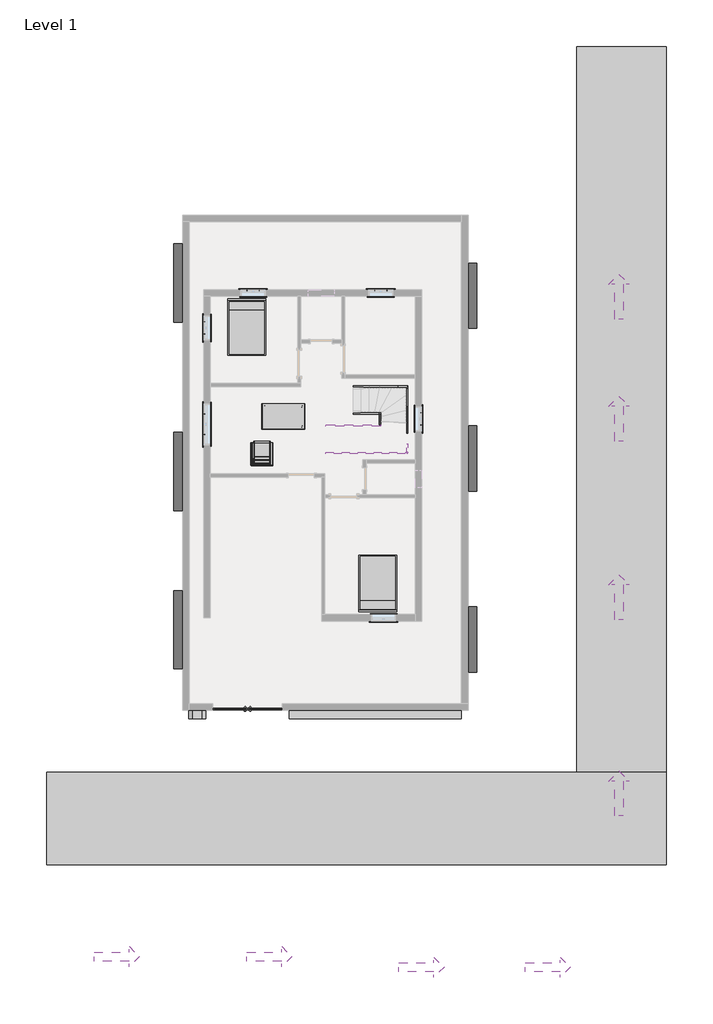
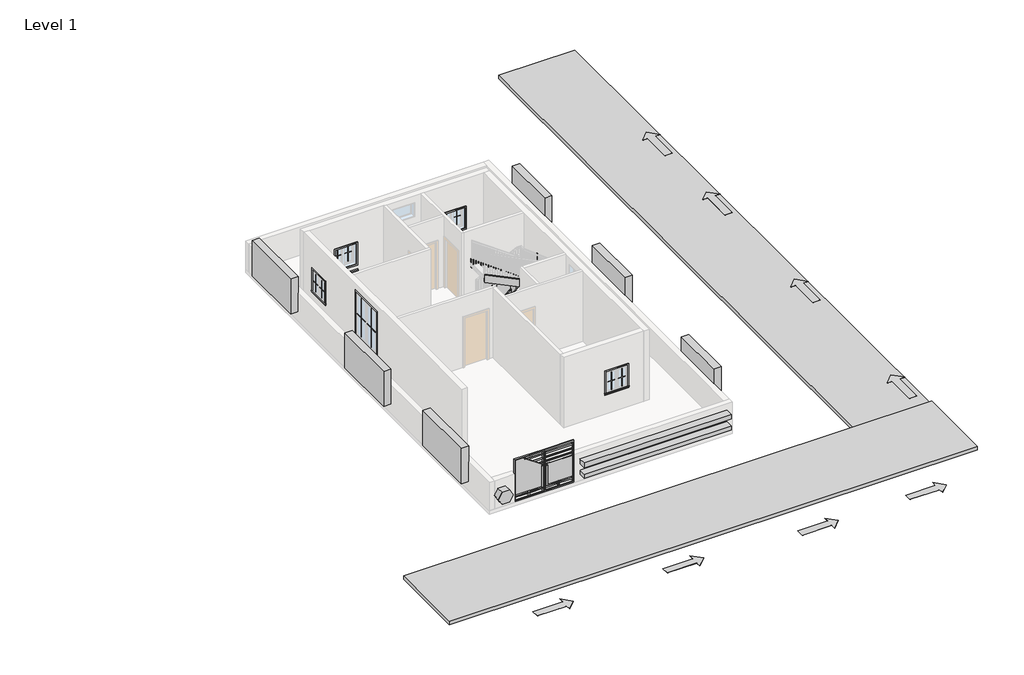
# One storey, part 3 of 3: 30 proxies, 9 members, 8 geographic elements, 4 furniture elements.
"""IFC4 building model written with IfcOpenShell, lengths in millimetres."""

from ifc_helpers import new_model, si_unit, frame, origin, place, context, project, spatial, polyline, outline, extrude, transform, mapped, element, save
from components import generic_models_113f6068, generic_models_1_generic_models_1_a47648ae, generic_models_2_generic_models_2_4eaefd90, generic_models_3_generic_models_3_d2748d51, generic_models_4_generic_models_4_994ceaf2, generic_models_5_generic_models_5_1652e53f, muntin_pattern_2x2_muntin_pattern_2x2_b3fe6957, muntin_pattern_2x2_muntin_pattern_2x2_3e0ecaf2, muntin_pattern_2x2_muntin_pattern_2x2_bff912c5, muntin_pattern_2x2_muntin_pattern_2x2_c2194282, trim_window_exterior_flat_with_sill_41619996, trim_window_exterior_flat_with_sill_e04b3088, trim_window_interior_flat_picture_frame_51c85655, trim_window_interior_flat_picture_frame_2a7685fe, furniture_f28dd14e, furniture_402a1f5e, bed_17739_bed_17739_15c61121, dining_table_14755_dining_table_14755_d89cb775, direction_arrows_straight_direction_arrow_straight_a0d3235c

model = new_model("IFC4")

# Units and contexts
model_context = context("Model", 3, world=origin())
ifc_project = project(units=[si_unit("LENGTHUNIT", "METRE", prefix="MILLI")], contexts=[model_context])

# Site, building, storey
site = spatial("IfcSite", under=ifc_project)
building = spatial("IfcBuilding", under=site)
storey = spatial("IfcBuildingStorey", under=building, Name="Level 1", Elevation=0.0)

# Proxies
placement = place(None, origin())
generic_models_shape = generic_models_113f6068(model_context)
element("IfcBuildingElementProxy", 1, Name="Generic Models", at=placement, inside=storey, context=model_context, shape_type="MappedRepresentation", body=[
    mapped(generic_models_shape, transform((-3534.8915084, -8307.1830082, 0.0), x_axis=(1.0, 0.0, 0.0), y_axis=(0.0, 1.0, 0.0), z_axis=(0.0, 0.0, 1.0))),
])
generic_models_1_generic_models_1_shape = generic_models_1_generic_models_1_a47648ae(model_context)
element("IfcBuildingElementProxy", 2, Name="Generic Models 1 : Generic Models 1", ObjectType="Generic Models 1 : Generic Models 1", at=placement, inside=storey, context=model_context, shape_type="MappedRepresentation", body=[
    mapped(generic_models_1_generic_models_1_shape, transform((0.0, 0.0, 0.0), x_axis=(1.0, 0.0, 0.0), y_axis=(0.0, 1.0, 0.0), z_axis=(0.0, 0.0, 1.0))),
])
generic_models_2_generic_models_2_shape = generic_models_2_generic_models_2_4eaefd90(model_context)
element("IfcBuildingElementProxy", 3, Name="Generic Models 2 : Generic Models 2", ObjectType="Generic Models 2 : Generic Models 2", at=placement, inside=storey, context=model_context, shape_type="MappedRepresentation", body=[
    mapped(generic_models_2_generic_models_2_shape, transform((0.0, 0.0, 0.0), x_axis=(1.0, 0.0, 0.0), y_axis=(0.0, 1.0, 0.0), z_axis=(0.0, 0.0, 1.0))),
])
generic_models_3_generic_models_3_shape = generic_models_3_generic_models_3_d2748d51(model_context)
element("IfcBuildingElementProxy", 4, Name="Generic Models 3 : Generic Models 3", ObjectType="Generic Models 3 : Generic Models 3", at=placement, inside=storey, context=model_context, shape_type="MappedRepresentation", body=[
    mapped(generic_models_3_generic_models_3_shape, transform((0.0, 0.0, 0.0), x_axis=(1.0, 0.0, 0.0), y_axis=(0.0, 1.0, 0.0), z_axis=(0.0, 0.0, 1.0))),
])
generic_models_4_generic_models_4_shape = generic_models_4_generic_models_4_994ceaf2(model_context)
element("IfcBuildingElementProxy", 5, Name="Generic Models 4 : Generic Models 4", ObjectType="Generic Models 4 : Generic Models 4", at=placement, inside=storey, context=model_context, shape_type="MappedRepresentation", body=[
    mapped(generic_models_4_generic_models_4_shape, transform((0.0, 0.0, 0.0), x_axis=(1.0, 0.0, 0.0), y_axis=(0.0, 1.0, 0.0), z_axis=(0.0, 0.0, 1.0))),
])
generic_models_5_generic_models_5_shape = generic_models_5_generic_models_5_1652e53f(model_context)
element("IfcBuildingElementProxy", 6, Name="Generic Models 5 : Generic Models 5", ObjectType="Generic Models 5 : Generic Models 5", at=placement, inside=storey, context=model_context, shape_type="MappedRepresentation", body=[
    mapped(generic_models_5_generic_models_5_shape, transform((0.0, 0.0, 0.0), x_axis=(1.0, 0.0, 0.0), y_axis=(0.0, 1.0, 0.0), z_axis=(0.0, 0.0, 1.0))),
])
muntin_pattern_2x2_muntin_pattern_2x2_shape = muntin_pattern_2x2_muntin_pattern_2x2_b3fe6957(model_context)
element("IfcBuildingElementProxy", 7, Name="Muntin Pattern_2x2 : Muntin Pattern_2x2", ObjectType="Muntin Pattern_2x2 : Muntin Pattern_2x2", at=placement, inside=storey, context=model_context, shape_type="MappedRepresentation", body=[
    mapped(muntin_pattern_2x2_muntin_pattern_2x2_shape, transform((-3555.5290084, 6319.8685985, 984.25), x_axis=(1.0, 0.0, 0.0), y_axis=(0.0, 1.0, 0.0), z_axis=(0.0, 0.0, 1.0))),
])
element("IfcBuildingElementProxy", 8, Name="Muntin Pattern_2x2 : Muntin Pattern_2x2", ObjectType="Muntin Pattern_2x2 : Muntin Pattern_2x2", at=placement, inside=storey, context=model_context, shape_type="MappedRepresentation", body=[
    mapped(muntin_pattern_2x2_muntin_pattern_2x2_shape, transform((1435.5709916, -5243.4814015, 984.25), x_axis=(-1.0, 0.0, 0.0), y_axis=(0.0, -1.0, 0.0), z_axis=(0.0, 0.0, 1.0))),
])
element("IfcBuildingElementProxy", 9, Name="Muntin Pattern_2x2 : Muntin Pattern_2x2", ObjectType="Muntin Pattern_2x2 : Muntin Pattern_2x2", at=placement, inside=storey, context=model_context, shape_type="MappedRepresentation", body=[
    mapped(muntin_pattern_2x2_muntin_pattern_2x2_shape, transform((2545.2334916, 2028.8560985, 984.25), x_axis=(0.0, -1.0, 0.0), y_axis=(1.0, 0.0, 0.0), z_axis=(0.0, 0.0, 1.0))),
])
element("IfcBuildingElementProxy", 10, Name="Muntin Pattern_2x2 : Muntin Pattern_2x2", ObjectType="Muntin Pattern_2x2 : Muntin Pattern_2x2", at=placement, inside=storey, context=model_context, shape_type="MappedRepresentation", body=[
    mapped(muntin_pattern_2x2_muntin_pattern_2x2_shape, transform((908.5209916, 6319.8685985, 984.25), x_axis=(1.0, 0.0, 0.0), y_axis=(0.0, 1.0, 0.0), z_axis=(0.0, 0.0, 1.0))),
])
element("IfcBuildingElementProxy", 11, Name="Muntin Pattern_2x2 : Muntin Pattern_2x2", ObjectType="Muntin Pattern_2x2 : Muntin Pattern_2x2", at=placement, inside=storey, context=model_context, shape_type="MappedRepresentation", body=[
    mapped(muntin_pattern_2x2_muntin_pattern_2x2_shape, transform((-5055.7165084, 4781.5810985, 984.25), x_axis=(0.0, 1.0, 0.0), y_axis=(-1.0, 0.0, 0.0), z_axis=(0.0, 0.0, 1.0))),
])
muntin_pattern_2x2_muntin_pattern_2x2_2_shape = muntin_pattern_2x2_muntin_pattern_2x2_3e0ecaf2(model_context)
element("IfcBuildingElementProxy", 12, Name="Muntin Pattern_2x2 : Muntin Pattern_2x2", ObjectType="Muntin Pattern_2x2 : Muntin Pattern_2x2", at=placement, inside=storey, context=model_context, shape_type="MappedRepresentation", body=[
    mapped(muntin_pattern_2x2_muntin_pattern_2x2_2_shape, transform((-3126.9040084, 6319.8685985, 984.25), x_axis=(-1.0, 0.0, 0.0), y_axis=(0.0, -1.0, 0.0), z_axis=(0.0, 0.0, 1.0))),
])
element("IfcBuildingElementProxy", 13, Name="Muntin Pattern_2x2 : Muntin Pattern_2x2", ObjectType="Muntin Pattern_2x2 : Muntin Pattern_2x2", at=placement, inside=storey, context=model_context, shape_type="MappedRepresentation", body=[
    mapped(muntin_pattern_2x2_muntin_pattern_2x2_2_shape, transform((1006.9459916, -5243.4814015, 984.25), x_axis=(1.0, 0.0, 0.0), y_axis=(0.0, 1.0, 0.0), z_axis=(0.0, 0.0, 1.0))),
])
element("IfcBuildingElementProxy", 14, Name="Muntin Pattern_2x2 : Muntin Pattern_2x2", ObjectType="Muntin Pattern_2x2 : Muntin Pattern_2x2", at=placement, inside=storey, context=model_context, shape_type="MappedRepresentation", body=[
    mapped(muntin_pattern_2x2_muntin_pattern_2x2_2_shape, transform((2545.2334916, 1600.2310985, 984.25), x_axis=(0.0, 1.0, 0.0), y_axis=(-1.0, 0.0, 0.0), z_axis=(0.0, 0.0, 1.0))),
])
element("IfcBuildingElementProxy", 15, Name="Muntin Pattern_2x2 : Muntin Pattern_2x2", ObjectType="Muntin Pattern_2x2 : Muntin Pattern_2x2", at=placement, inside=storey, context=model_context, shape_type="MappedRepresentation", body=[
    mapped(muntin_pattern_2x2_muntin_pattern_2x2_2_shape, transform((1337.1459916, 6319.8685985, 984.25), x_axis=(-1.0, 0.0, 0.0), y_axis=(0.0, -1.0, 0.0), z_axis=(0.0, 0.0, 1.0))),
])
element("IfcBuildingElementProxy", 16, Name="Muntin Pattern_2x2 : Muntin Pattern_2x2", ObjectType="Muntin Pattern_2x2 : Muntin Pattern_2x2", at=placement, inside=storey, context=model_context, shape_type="MappedRepresentation", body=[
    mapped(muntin_pattern_2x2_muntin_pattern_2x2_2_shape, transform((-5055.7165084, 5210.2060985, 984.25), x_axis=(0.0, -1.0, 0.0), y_axis=(1.0, 0.0, 0.0), z_axis=(0.0, 0.0, 1.0))),
])
muntin_pattern_2x2_muntin_pattern_2x2_3_shape = muntin_pattern_2x2_muntin_pattern_2x2_bff912c5(model_context)
element("IfcBuildingElementProxy", 17, Name="Muntin Pattern_2x2 : Muntin Pattern_2x2", ObjectType="Muntin Pattern_2x2 : Muntin Pattern_2x2", at=placement, inside=storey, context=model_context, shape_type="MappedRepresentation", body=[
    mapped(muntin_pattern_2x2_muntin_pattern_2x2_3_shape, transform((-5055.7165084, 1263.6810985, 984.25), x_axis=(0.0, 1.0, 0.0), y_axis=(-1.0, 0.0, 0.0), z_axis=(0.0, 0.0, 1.0))),
])
muntin_pattern_2x2_muntin_pattern_2x2_4_shape = muntin_pattern_2x2_muntin_pattern_2x2_c2194282(model_context)
element("IfcBuildingElementProxy", 18, Name="Muntin Pattern_2x2 : Muntin Pattern_2x2", ObjectType="Muntin Pattern_2x2 : Muntin Pattern_2x2", at=placement, inside=storey, context=model_context, shape_type="MappedRepresentation", body=[
    mapped(muntin_pattern_2x2_muntin_pattern_2x2_4_shape, transform((-5055.7165084, 1984.4060985, 984.25), x_axis=(0.0, -1.0, 0.0), y_axis=(1.0, 0.0, 0.0), z_axis=(0.0, 0.0, 1.0))),
])
trim_window_exterior_flat_with_sill_shape = trim_window_exterior_flat_with_sill_41619996(model_context)
element("IfcBuildingElementProxy", 19, Name="Trim-Window-Exterior-Flat : with Sill", ObjectType="Trim-Window-Exterior-Flat : with Sill", at=placement, inside=storey, context=model_context, shape_type="MappedRepresentation", body=[
    mapped(trim_window_exterior_flat_with_sill_shape, transform((-3341.2165084, 6329.3935985, 1828.8), x_axis=(-1.0, 0.0, 0.0), y_axis=(0.0, 0.0, 1.0), z_axis=(0.0, 1.0, 0.0))),
])
element("IfcBuildingElementProxy", 20, Name="Trim-Window-Exterior-Flat : with Sill", ObjectType="Trim-Window-Exterior-Flat : with Sill", at=placement, inside=storey, context=model_context, shape_type="MappedRepresentation", body=[
    mapped(trim_window_exterior_flat_with_sill_shape, transform((1221.2584916, -5253.0064015, 1828.8), x_axis=(1.0, 0.0, 0.0), y_axis=(0.0, 0.0, 1.0), z_axis=(0.0, -1.0, 0.0))),
])
element("IfcBuildingElementProxy", 21, Name="Trim-Window-Exterior-Flat : with Sill", ObjectType="Trim-Window-Exterior-Flat : with Sill", at=placement, inside=storey, context=model_context, shape_type="MappedRepresentation", body=[
    mapped(trim_window_exterior_flat_with_sill_shape, transform((2554.7584916, 1814.5435985, 1828.8), x_axis=(0.0, 1.0, 0.0), y_axis=(0.0, 0.0, 1.0), z_axis=(1.0, 0.0, 0.0))),
])
element("IfcBuildingElementProxy", 22, Name="Trim-Window-Exterior-Flat : with Sill", ObjectType="Trim-Window-Exterior-Flat : with Sill", at=placement, inside=storey, context=model_context, shape_type="MappedRepresentation", body=[
    mapped(trim_window_exterior_flat_with_sill_shape, transform((1122.8334916, 6329.3935985, 1828.8), x_axis=(-1.0, 0.0, 0.0), y_axis=(0.0, 0.0, 1.0), z_axis=(0.0, 1.0, 0.0))),
])
element("IfcBuildingElementProxy", 23, Name="Trim-Window-Exterior-Flat : with Sill", ObjectType="Trim-Window-Exterior-Flat : with Sill", at=placement, inside=storey, context=model_context, shape_type="MappedRepresentation", body=[
    mapped(trim_window_exterior_flat_with_sill_shape, transform((-5065.2415084, 4995.8935985, 1828.8), x_axis=(0.0, -1.0, 0.0), y_axis=(0.0, 0.0, 1.0), z_axis=(-1.0, 0.0, 0.0))),
])
trim_window_exterior_flat_with_sill_2_shape = trim_window_exterior_flat_with_sill_e04b3088(model_context)
element("IfcBuildingElementProxy", 24, Name="Trim-Window-Exterior-Flat : with Sill", ObjectType="Trim-Window-Exterior-Flat : with Sill", at=placement, inside=storey, context=model_context, shape_type="MappedRepresentation", body=[
    mapped(trim_window_exterior_flat_with_sill_2_shape, transform((-5065.2415084, 1624.0435985, 2743.2), x_axis=(0.0, -1.0, 0.0), y_axis=(0.0, 0.0, 1.0), z_axis=(-1.0, 0.0, 0.0))),
])
trim_window_interior_flat_picture_frame_shape = trim_window_interior_flat_picture_frame_51c85655(model_context)
element("IfcBuildingElementProxy", 25, Name="Trim-Window-Interior-Flat : Picture Frame", ObjectType="Trim-Window-Interior-Flat : Picture Frame", at=placement, inside=storey, context=model_context, shape_type="MappedRepresentation", body=[
    mapped(trim_window_interior_flat_picture_frame_shape, transform((-3341.2165084, 6100.7935985, 1828.8), x_axis=(1.0, 0.0, 0.0), y_axis=(0.0, 0.0, 1.0), z_axis=(0.0, -1.0, 0.0))),
])
element("IfcBuildingElementProxy", 26, Name="Trim-Window-Interior-Flat : Picture Frame", ObjectType="Trim-Window-Interior-Flat : Picture Frame", at=placement, inside=storey, context=model_context, shape_type="MappedRepresentation", body=[
    mapped(trim_window_interior_flat_picture_frame_shape, transform((1221.2584916, -5024.4064015, 1828.8), x_axis=(-1.0, 0.0, 0.0), y_axis=(0.0, 0.0, 1.0), z_axis=(0.0, 1.0, 0.0))),
])
element("IfcBuildingElementProxy", 27, Name="Trim-Window-Interior-Flat : Picture Frame", ObjectType="Trim-Window-Interior-Flat : Picture Frame", at=placement, inside=storey, context=model_context, shape_type="MappedRepresentation", body=[
    mapped(trim_window_interior_flat_picture_frame_shape, transform((2326.1584916, 1814.5435985, 1828.8), x_axis=(0.0, -1.0, 0.0), y_axis=(0.0, 0.0, 1.0), z_axis=(-1.0, 0.0, 0.0))),
])
element("IfcBuildingElementProxy", 28, Name="Trim-Window-Interior-Flat : Picture Frame", ObjectType="Trim-Window-Interior-Flat : Picture Frame", at=placement, inside=storey, context=model_context, shape_type="MappedRepresentation", body=[
    mapped(trim_window_interior_flat_picture_frame_shape, transform((1122.8334916, 6100.7935985, 1828.8), x_axis=(1.0, 0.0, 0.0), y_axis=(0.0, 0.0, 1.0), z_axis=(0.0, -1.0, 0.0))),
])
element("IfcBuildingElementProxy", 29, Name="Trim-Window-Interior-Flat : Picture Frame", ObjectType="Trim-Window-Interior-Flat : Picture Frame", at=placement, inside=storey, context=model_context, shape_type="MappedRepresentation", body=[
    mapped(trim_window_interior_flat_picture_frame_shape, transform((-4836.6415084, 4995.8935985, 1828.8), x_axis=(0.0, 1.0, 0.0), y_axis=(0.0, 0.0, 1.0), z_axis=(1.0, 0.0, 0.0))),
])
trim_window_interior_flat_picture_frame_2_shape = trim_window_interior_flat_picture_frame_2a7685fe(model_context)
element("IfcBuildingElementProxy", 30, Name="Trim-Window-Interior-Flat : Picture Frame", ObjectType="Trim-Window-Interior-Flat : Picture Frame", at=placement, inside=storey, context=model_context, shape_type="MappedRepresentation", body=[
    mapped(trim_window_interior_flat_picture_frame_2_shape, transform((-4836.6415084, 1624.0435985, 2743.2), x_axis=(0.0, 1.0, 0.0), y_axis=(0.0, 0.0, 1.0), z_axis=(1.0, 0.0, 0.0))),
])

# Furniture
furniture_shape = furniture_f28dd14e(model_context)
furniture_2_shape = furniture_402a1f5e(model_context)
element("IfcFurniture", 31, at=placement, inside=storey, context=model_context, shape_type="MappedRepresentation", body=[
    mapped(furniture_shape, transform((-3032.3877006, 981.9349825, 0.0), x_axis=(-1.0, 0.0, 0.0), y_axis=(0.0, -1.0, 0.0), z_axis=(0.0, 0.0, 1.0))),
    mapped(furniture_2_shape, transform((-3032.3877006, 981.9349825, 0.0), x_axis=(-1.0, 0.0, 0.0), y_axis=(0.0, -1.0, 0.0), z_axis=(0.0, 0.0, 1.0))),
])
bed_17739_bed_17739_shape = bed_17739_bed_17739_15c61121(model_context)
element("IfcFurniture", 32, ObjectType="Bed_17739 : Bed_17739", at=placement, inside=storey, context=model_context, shape_type="MappedRepresentation", body=[
    mapped(bed_17739_bed_17739_shape, transform((-3560.2915084, 4995.8935985, 0.0), x_axis=(1.0, 0.0, 0.0), y_axis=(0.0, 1.0, 0.0), z_axis=(0.0, 0.0, 1.0))),
])
element("IfcFurniture", 33, ObjectType="Bed_17739 : Bed_17739", at=placement, inside=storey, context=model_context, shape_type="MappedRepresentation", body=[
    mapped(bed_17739_bed_17739_shape, transform((1011.7084916, -3919.5064015, 0.0), x_axis=(-1.0, 0.0, 0.0), y_axis=(0.0, -1.0, 0.0), z_axis=(0.0, 0.0, 1.0))),
])
dining_table_14755_dining_table_14755_shape = dining_table_14755_dining_table_14755_d89cb775(model_context)
element("IfcFurniture", 34, ObjectType="Dining_table_14755 : Dining_table_14755", at=placement, inside=storey, context=model_context, shape_type="MappedRepresentation", body=[
    mapped(dining_table_14755_dining_table_14755_shape, transform((-3032.3877006, 1444.8879061, 0.0), x_axis=(1.0, 0.0, 0.0), y_axis=(0.0, 1.0, 0.0), z_axis=(0.0, 0.0, 1.0))),
])

# Geographic elements
direction_arrows_straight_direction_arrow_straight_shape = direction_arrows_straight_direction_arrow_straight_a0d3235c(model_context)
element("IfcGeographicElement", 35, ObjectType="Direction Arrows - Straight : Direction Arrow - Straight", at=placement, inside=storey, context=model_context, shape_type="MappedRepresentation", body=[
    mapped(direction_arrows_straight_direction_arrow_straight_shape, transform((-8896.9922047, -16987.8064015, 1828.8), x_axis=(0.0, -1.0, 0.0), y_axis=(1.0, 0.0, 0.0), z_axis=(0.0, 0.0, 1.0))),
])
element("IfcGeographicElement", 36, ObjectType="Direction Arrows - Straight : Direction Arrow - Straight", at=placement, inside=storey, context=model_context, shape_type="MappedRepresentation", body=[
    mapped(direction_arrows_straight_direction_arrow_straight_shape, transform((-3562.9922047, -16987.8064015, 1828.8), x_axis=(0.0, -1.0, 0.0), y_axis=(1.0, 0.0, 0.0), z_axis=(0.0, 0.0, 1.0))),
])
element("IfcGeographicElement", 37, ObjectType="Direction Arrows - Straight : Direction Arrow - Straight", at=placement, inside=storey, context=model_context, shape_type="MappedRepresentation", body=[
    mapped(direction_arrows_straight_direction_arrow_straight_shape, transform((1758.0144394, -17359.8874325, 1828.8), x_axis=(0.0, -1.0, 0.0), y_axis=(1.0, 0.0, 0.0), z_axis=(0.0, 0.0, 1.0))),
])
element("IfcGeographicElement", 38, ObjectType="Direction Arrows - Straight : Direction Arrow - Straight", at=placement, inside=storey, context=model_context, shape_type="MappedRepresentation", body=[
    mapped(direction_arrows_straight_direction_arrow_straight_shape, transform((6177.6144394, -17359.8874325, 1828.8), x_axis=(0.0, -1.0, 0.0), y_axis=(1.0, 0.0, 0.0), z_axis=(0.0, 0.0, 1.0))),
])
element("IfcGeographicElement", 39, ObjectType="Direction Arrows - Straight : Direction Arrow - Straight", at=placement, inside=storey, context=model_context, shape_type="MappedRepresentation", body=[
    mapped(direction_arrows_straight_direction_arrow_straight_shape, transform((9447.5076868, -12069.3629782, 1828.8), x_axis=(1.0, 0.0, 0.0), y_axis=(0.0, 1.0, 0.0), z_axis=(0.0, 0.0, 1.0))),
])
element("IfcGeographicElement", 40, ObjectType="Direction Arrows - Straight : Direction Arrow - Straight", at=placement, inside=storey, context=model_context, shape_type="MappedRepresentation", body=[
    mapped(direction_arrows_straight_direction_arrow_straight_shape, transform((9447.5076868, -5211.3629782, 1828.8), x_axis=(1.0, 0.0, 0.0), y_axis=(0.0, 1.0, 0.0), z_axis=(0.0, 0.0, 1.0))),
])
element("IfcGeographicElement", 41, ObjectType="Direction Arrows - Straight : Direction Arrow - Straight", at=placement, inside=storey, context=model_context, shape_type="MappedRepresentation", body=[
    mapped(direction_arrows_straight_direction_arrow_straight_shape, transform((9447.5076868, 1037.0370218, 1828.8), x_axis=(1.0, 0.0, 0.0), y_axis=(0.0, 1.0, 0.0), z_axis=(0.0, 0.0, 1.0))),
])
element("IfcGeographicElement", 42, ObjectType="Direction Arrows - Straight : Direction Arrow - Straight", at=placement, inside=storey, context=model_context, shape_type="MappedRepresentation", body=[
    mapped(direction_arrows_straight_direction_arrow_straight_shape, transform((9447.5076868, 5304.2370218, 1828.8), x_axis=(1.0, 0.0, 0.0), y_axis=(0.0, 1.0, 0.0), z_axis=(0.0, 0.0, 1.0))),
])

# Members
element("IfcMember", 43, ObjectType="Stringer - 2\" Width", at=placement, inside=storey, context=model_context, shape_type="SweptSolid", body=[
    extrude(outline(polyline([(239.4504763, 158.6923968), (0.0, 158.6923968), (0.0, 366.2169505), (626.2639814, 1705.9967367), (962.7193197, 1705.9967367), (239.4504763, 158.6923968)])), frame((0.0, 2922.8476133, 0.0), z_axis=(0.0, 1.0, 0.0), x_axis=(0.0, 0.0, 1.0)), (0.0, 0.0, 1.0), 50.8),
])
element("IfcMember", 44, ObjectType="Stringer - 2\" Width", at=placement, inside=storey, context=model_context, shape_type="SweptSolid", body=[
    extrude(outline(polyline([(1705.9967367, 2922.8476133), (1705.9967367, 2973.6476133), (2072.9441983, 2973.6476133), (2022.1441983, 2922.8476133), (1705.9967367, 2922.8476133)])), frame((0.0, 0.0, 626.2639814), z_axis=(0.0, 0.0, 1.0), x_axis=(1.0, 0.0, 0.0)), (0.0, 0.0, 1.0), 336.4553383),
])
element("IfcMember", 45, ObjectType="Stringer - 2\" Width", at=placement, inside=storey, context=model_context, shape_type="SweptSolid", body=[
    extrude(outline(polyline([(2022.1441983, 2922.8476133), (2072.9441983, 2973.6476133), (2072.9441983, 2883.4348143), (2022.1441983, 2883.4348143), (2022.1441983, 2922.8476133)])), frame((0.0, 0.0, 626.2639814), z_axis=(0.0, 0.0, 1.0), x_axis=(1.0, 0.0, 0.0)), (0.0, 0.0, 1.0), 336.4553383),
])
element("IfcMember", 46, ObjectType="Stringer - 2\" Width", at=placement, inside=storey, context=model_context, shape_type="SweptSolid", body=[
    extrude(outline(polyline([(2883.4348143, 962.7193197), (2883.4348143, 626.2639814), (947.0260734, 1335.6990218), (947.0260734, 1672.1543601), (2883.4348143, 962.7193197)])), frame((2022.1441983, 0.0, 0.0), z_axis=(1.0, 0.0, 0.0), x_axis=(0.0, 1.0, 0.0)), (0.0, 0.0, 1.0), 50.8),
])
element("IfcMember", 47, ObjectType="Stringer - 2\" Width", at=placement, inside=storey, context=model_context, shape_type="SweptSolid", body=[
    extrude(outline(polyline([(2022.1441983, 947.0260734), (2072.9441983, 947.0260734), (2072.9441983, 652.4935985), (2022.1441983, 652.4935985), (2022.1441983, 947.0260734)])), frame((0.0, 0.0, 1341.3754285), z_axis=(0.0, 0.0, 1.0), x_axis=(1.0, 0.0, 0.0)), (0.0, 0.0, 1.0), 324.6119022),
])
element("IfcMember", 48, ObjectType="Stringer - 2\" Width", at=placement, inside=storey, context=model_context, shape_type="SweptSolid", body=[
    extrude(outline(polyline([(174.4551137, 158.6923968), (0.0, 158.6923968), (0.0, 426.0767146), (534.1870321, 1072.5901835), (929.5706215, 1072.5901835), (174.4551137, 158.6923968)])), frame((0.0, 1973.2935985, 0.0), z_axis=(0.0, 1.0, 0.0), x_axis=(0.0, 0.0, 1.0)), (0.0, 0.0, 1.0), 50.8),
])
element("IfcMember", 49, ObjectType="Stringer - 2\" Width", at=placement, inside=storey, context=model_context, shape_type="SweptSolid", body=[
    extrude(outline(polyline([(2024.0935985, 1132.896008), (2024.0935985, 630.1724164), (1602.0476133, 1183.7407029), (1602.0476133, 1686.4642945), (2024.0935985, 1132.896008)])), frame((1072.5901835, 0.0, 0.0), z_axis=(1.0, 0.0, 0.0), x_axis=(0.0, 1.0, 0.0)), (0.0, 0.0, 1.0), 50.8),
])
element("IfcMember", 50, ObjectType="Stringer - 2\" Width", at=placement, inside=storey, context=model_context, shape_type="SweptSolid", body=[
    extrude(outline(polyline([(1362.1113348, 1123.3901835), (1739.0379401, 1123.3901835), (3137.1009734, -798.3242294), (2760.1743681, -798.3242294), (1362.1113348, 1123.3901835)])), frame((0.0, 1551.2476133, 0.0), z_axis=(0.0, 1.0, 0.0), x_axis=(0.0, 0.0, 1.0)), (0.0, 0.0, 1.0), 50.8),
])
element("IfcMember", 51, ObjectType="Stringer - 2\" Width", at=placement, inside=storey, context=model_context, shape_type="SweptSolid", body=[
    extrude(outline(polyline([(1361.1873308, 2072.9441983), (1641.2397747, 2072.9441983), (3039.9971818, -798.3242294), (2715.3852796, -798.3242294), (1361.1873308, 1981.4757528), (1361.1873308, 2072.9441983)])), frame((0.0, 601.6935985, 0.0), z_axis=(0.0, 1.0, 0.0), x_axis=(0.0, 0.0, 1.0)), (0.0, 0.0, 1.0), 50.8),
])

save(model, "model.ifc")

# Revit data of these elements
# Type
#   sheet = none
#   pipe = none
#   handal = none
#   faram = none
#   Default Elevation = 0
# Type "Muntin Pattern_2x2 : Muntin Pattern_2x2"
#   Width [instance default] = 4' - 0"
#   Thickness = 0' - 0 1/2"
#   Height [instance default] = 4' - 0"
#   Distance = 0' - 0 3/4"
#   Interior Material [instance default] = none
#   Exterior Material [instance default] = none
#   Default Elevation = 0
# Type "Trim-Window-Exterior-Flat : with Sill"
#   Trim Width = 0' - 2 1/4"
#   Trim Thickness_Picture Frame = 0' - 1 1/4"
#   Trim Thickness_with Sill = 0' - 0 3/4"
#   Sill Thickness = 0' - 1 1/4"
#   Opening Width [instance default] = 2' - 0"
#   Opening Height [instance default] = 3' - 0"
#   Default Elevation = 4' - 0"
#   Sill = yes
#   Picture Frame = no
#   Trim Material [instance default] = none
# Type "Trim-Window-Interior-Flat : Picture Frame"
#   Trim Thickness_Picture Frame = 0' - 1 1/4"
#   Trim Width = 0' - 2 1/4"
#   Trim Thickness_with Sill = 0' - 0 3/4"
#   Sill Thickness = 0' - 1 1/4"
#   Opening Width [instance default] = 2' - 0"
#   Opening Height [instance default] = 3' - 0"
#   Default Elevation = 4' - 0"
#   Sill = no
#   Picture Frame = yes
#   Trim Material [instance default] = none
# Type
#   Width [instance] = 2' - 6.31496"
#   Default Elevation = 0
# Type "Bed_17739 : Bed_17739"
#   Default Elevation = 0
# Type "Dining_table_14755 : Dining_table_14755"
#   Lengte [instance default] = 4' - 11.05512"
#   Breedte [instance default] = 2' - 11.43307"
#   Tafelblad = none
#   Poten = none
#   Default Elevation = 0
# Element 1 (IfcBuildingElementProxy)
#   Phase Created = New Construction
# Element 2 (IfcBuildingElementProxy, "Generic Models 1 : Generic Models 1")
#   Phase Created = New Construction
#   Materials on its faces: "Wood - Stained", "Softwood, Lumber"
# Element 3 (IfcBuildingElementProxy, "Generic Models 2 : Generic Models 2")
#   Phase Created = New Construction
#   Materials on its faces: "Wood - Stained"
# Element 4 (IfcBuildingElementProxy, "Generic Models 3 : Generic Models 3")
#   Phase Created = New Construction
#   Materials on its faces: "Parking Stripe"
# Element 5 (IfcBuildingElementProxy, "Generic Models 4 : Generic Models 4")
#   Phase Created = New Construction
#   Materials on its faces: "Parking Stripe"
# Element 6 (IfcBuildingElementProxy, "Generic Models 5 : Generic Models 5")
#   Phase Created = New Construction
# Elements 7, 8, 9, 10, 11, 12, 13, 14, 15, 16 (IfcBuildingElementProxy, "Muntin Pattern_2x2 : Muntin Pattern_2x2")
#   Width = 0' - 11 5/8"
#   Height = 2' - 6 1/2"
#   Interior Material = Wood - Stained
#   Exterior Material = Clad - White
#   Phase Created = New Construction
#   Materials on its faces: "Clad - White", "Wood - Stained"
# Elements 17, 18 (IfcBuildingElementProxy, "Muntin Pattern_2x2 : Muntin Pattern_2x2")
#   Width = 1' - 11 1/8"
#   Height = 5' - 6 1/2"
#   Interior Material = Wood - Stained
#   Exterior Material = Clad - White
#   Phase Created = New Construction
#   Materials on its faces: "Clad - White", "Wood - Stained"
# Elements 19, 20, 21, 22, 23 (IfcBuildingElementProxy, "Trim-Window-Exterior-Flat : with Sill")
#   Opening Width = 2' - 10"
#   Opening Height = 3' - 0"
#   Trim Material = Clad - White
#   Phase Created = New Construction
#   Materials on its faces: "Clad - White"
# Element 24 (IfcBuildingElementProxy, "Trim-Window-Exterior-Flat : with Sill")
#   Opening Width = 4' - 9"
#   Opening Height = 6' - 0"
#   Trim Material = Clad - White
#   Phase Created = New Construction
#   Materials on its faces: "Clad - White"
# Elements 25, 26, 27, 28, 29 (IfcBuildingElementProxy, "Trim-Window-Interior-Flat : Picture Frame")
#   Opening Width = 2' - 10"
#   Opening Height = 3' - 0"
#   Trim Material = Wood - Stained
#   Phase Created = New Construction
#   Materials on its faces: "Wood - Stained"
# Element 30 (IfcBuildingElementProxy, "Trim-Window-Interior-Flat : Picture Frame")
#   Opening Width = 4' - 9"
#   Opening Height = 6' - 0"
#   Trim Material = Wood - Stained
#   Phase Created = New Construction
#   Materials on its faces: "Wood - Stained"
# Element 31 (IfcFurniture)
#   Width = 2' - 6.31496"
#   Phase Created = New Construction
# Elements 32, 33 (IfcFurniture, "Bed_17739 : Bed_17739")
#   Phase Created = New Construction
#   Materials on its faces: "legs", "sheets", "bed frame", "Blanket"
# Element 34 (IfcFurniture, "Dining_table_14755 : Dining_table_14755")
#   Lengte = 4' - 11.05512"
#   Breedte = 2' - 11.43307"
#   Phase Created = New Construction
# Elements 35, 36, 37, 38, 39, 40, 41, 42 (IfcGeographicElement, "Direction Arrows - Straight : Direction Arrow - Straight")
#   Phase Created = New Construction
#   Materials on its faces: "Paint - White"
# Elements 43, 44, 45, 46, 47, 48, 49, 50, 51 (IfcMember, "Stringer - 2\" Width")
#   Phase Created = New Construction
# Materials
#   "Wood - Stained": class "Wood", colour RGB 224 178 126, transparency 0, Cost = 0
#   "Softwood, Lumber": class "Wood", colour RGB 223 192 134, transparency 0, Description = "Pinus Echinata", Cost = 0
#   "Parking Stripe": class "Paint", colour RGB 250 250 91, transparency 0, Cost = 0
#   "Clad - White": class "Wood", colour RGB 242 242 238, transparency 0, Cost = 0
#   "legs": colour RGB 90 73 37, transparency 0, Cost = 0
#   "sheets": colour RGB 200 195 176, transparency 0, Cost = 0
#   "bed frame": colour RGB 90 73 37, transparency 0, Cost = 0
#   "Blanket": class "System", colour RGB 59 0 1, transparency 0, Cost = 0
#   "Paint - White": class "Paint", colour RGB 249 249 249, transparency 0
